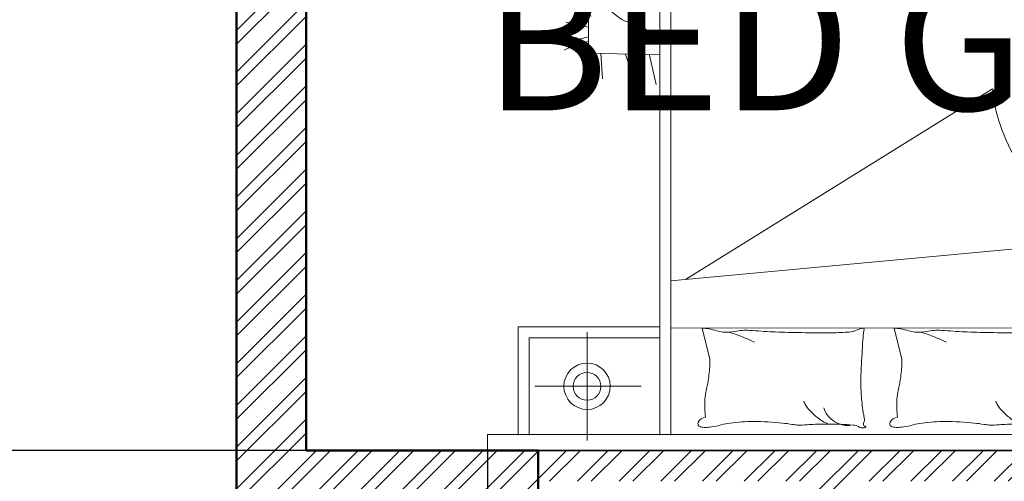
# Model space of a CAD drawing. Units: inches. Extents: x -90 to 536, y -553 to 299.
# Tile 17 of 27: x 10 to 137, y -2 to 58. Entities that reach past the tile are written whole.
import ezdxf

# ---------------------------------------------------------------- set-up
doc = ezdxf.new("R2010")
doc.units = ezdxf.units.IN
for name, color, linetype, lineweight in [('A-ANNO-DIMS', 2, 'Continuous', 18), ('A-WALL-PATT', 252, 'Continuous', 13), ('Furniture', 2, 'Continuous', 18), ('Inner Wall', 5, 'Continuous', 35), ('Outer Wall', 1, 'Continuous', 50)]:
    doc.layers.add(name, color=color, linetype=linetype, lineweight=lineweight)
doc.styles.get("Standard").update_dxf_attribs({"font": 'arial.ttf'})
doc.dimstyles.get("Standard").update_dxf_attribs({"dimtxt": 18, "dimasz": 12, "dimexe": 0.18, "dimexo": 0.0625, "dimgap": 0.09, "dimtad": 0, "dimtih": 1, "dimtoh": 1, "dimdec": 0, "dimzin": 0, "dimdsep": 46, "dimlunit": 3, "dimtxsty": 'Standard', "dimcen": 0.09, "dimadec": 0, "dimazin": 0, "dimtfac": 1, "dimtdec": 0, "dimtofl": 0, "dimtmove": 0, "dimatfit": 3, "dimfxl": 1, "dimtolj": 1, "dimtzin": 0, "dimarcsym": 0})

# ---------------------------------------------------------------- blocks, each defined once
blk = doc.blocks.new('A$C2B723114')
for p, q in [((0, 2.9047), (2.8274, 2.9047)), ((0, 2.8487), (0, 2.9047)), ((2.8274, 2.9047), (2.8274, 2.8487)), ((0.4243, 2.8697), (0.4243, 2.4855)), ((2.4742, 2.8697), (2.4742, 2.4855)), ((2.8274, 2.8487), (0, 2.8487)), ((0.1012, 2.4649), (0.1012, 2.849)), ((0.1396, 2.5033), (0.1396, 2.849)), ((0.6794, 0.7051), (0.6794, 2.8509)), ((0.7187, 0.7435), (0.7187, 2.8509)), ((2.1776, 2.8509), (2.1776, 0.7454)), ((2.216, 2.8509), (2.216, 0.707)), ((2.6798, 2.5052), (2.6798, 2.8509)), ((2.7182, 2.4668), (2.7182, 2.8509)), ((0.6087, 2.6776), (0.295, 2.6776)), ((2.6586, 2.6776), (2.2821, 2.6776)), ((1.3789, 2.4999), (1.3598, 2.5761)), ((2.0593, 2.4999), (2.0402, 2.5761)), ((0.6766, 2.5033), (0.1396, 2.5033)), ((1.3858, 2.4723), (1.3789, 2.4999)), ((2.0662, 2.4723), (2.0593, 2.4999)), ((2.2188, 2.5052), (2.6798, 2.5052)), ((0.6794, 2.4649), (0.1012, 2.4649)), ((0.7191, 2.47), (2.1778, 2.4719)), ((2.2188, 2.4668), (2.7182, 2.4668)), ((2.1771, 2.3036), (0.718, 2.1685)), ((1.0365, 1.6233), (2.1246, 2.2989)), ((2.2287, 1.6076), (2.2523, 1.5035)), ((0.5047, 1.5819), (0.5353, 1.4945)), ((0.6174, 1.5819), (0.6232, 1.4916)), ((0.6467, 1.5819), (0.6369, 1.5137)), ((0.6571, 1.4945), (0.6571, 1.5765)), ((2.2726, 1.593), (2.3061, 1.5007)), ((2.3067, 1.5881), (2.3373, 1.5007)), ((2.4194, 1.5881), (2.4251, 1.4979)), ((2.4487, 1.5881), (2.4389, 1.5199)), ((2.4591, 1.5007), (2.4591, 1.5828)), ((2.4685, 1.4964), (2.216, 1.5022)), ((0.4269, 0.0884), (0.4269, 1.4945)), ((0.4269, 1.4945), (0.6794, 1.4945)), ((2.4685, 1.4964), (2.4685, 0.0903)), ((2.4685, 1.4044), (2.5491, 1.3861)), ((0.3172, 1.3923), (0.4213, 1.3687)), ((2.4596, 1.3659), (2.552, 1.3324)), ((0.3318, 1.3485), (0.4241, 1.3149)), ((2.4645, 1.3318), (2.552, 1.3012)), ((0.3367, 1.3143), (0.4241, 1.2838)), ((2.4645, 1.2928), (2.5548, 1.2871)), ((2.4645, 1.2635), (2.5328, 1.2733)), ((2.4699, 1.2531), (2.552, 1.2163)), ((2.552, 1.2531), (2.4699, 1.2531)), ((2.5435, 1.2276), (2.4699, 1.2163)), ((0.3367, 1.2016), (0.427, 1.1959)), ((2.4699, 1.2163), (2.5463, 1.1823)), ((0.3367, 1.1724), (0.405, 1.1821)), ((0.4241, 1.162), (0.3421, 1.162)), ((0.3421, 1.162), (0.4241, 1.1252)), ((2.5491, 1.1654), (2.467, 1.1597)), ((2.5463, 1.1455), (2.467, 1.1342)), ((2.5491, 1.1342), (2.4699, 1.1201)), ((2.4699, 1.1201), (2.5491, 1.0946)), ((2.5463, 1.1172), (2.4727, 1.0918)), ((2.5491, 1.0946), (2.4699, 1.0635)), ((2.4699, 1.0635), (2.5491, 0.9842)), ((0.4157, 1.0206), (0.3421, 1.0093)), ((2.4642, 1.0267), (2.552, 0.9644)), ((0.3421, 1.0093), (0.4185, 0.9754)), ((2.4699, 0.9785), (2.552, 0.9531)), ((0.4213, 0.9584), (0.3392, 0.9527)), ((2.467, 0.9559), (2.552, 0.9333)), ((0.4185, 0.9386), (0.3392, 0.9272)), ((0.4213, 0.9272), (0.3421, 0.9131)), ((0.3421, 0.9131), (0.4213, 0.8876)), ((0.4185, 0.9103), (0.3449, 0.8848)), ((2.4642, 0.9389), (2.4869, 0.9276)), ((2.4869, 0.9276), (2.5265, 0.9163)), ((2.5265, 0.9163), (2.5491, 0.9163)), ((0.4213, 0.8876), (0.3421, 0.8565)), ((2.4642, 0.8908), (2.5152, 0.8483)), ((0.3421, 0.8565), (0.4213, 0.7772)), ((2.467, 0.8455), (2.5208, 0.8342)), ((2.5152, 0.8483), (2.5491, 0.837)), ((0.3364, 0.8197), (0.4241, 0.7574)), ((2.4699, 0.8172), (2.4925, 0.7974)), ((2.5491, 0.8087), (2.4699, 0.8172)), ((2.5208, 0.8342), (2.552, 0.8285)), ((2.552, 0.8285), (2.5293, 0.8087)), ((0.3421, 0.7716), (0.4241, 0.7461)), ((2.5491, 0.7606), (2.467, 0.7719)), ((2.4925, 0.7974), (2.535, 0.7889)), ((2.535, 0.7889), (2.552, 0.7861)), ((0.3392, 0.7489), (0.4241, 0.7263)), ((2.1776, 0.7454), (0.7187, 0.7435)), ((2.4727, 0.7464), (2.467, 0.7408)), ((2.552, 0.7464), (2.4727, 0.7464)), ((0.359, 0.7206), (0.3987, 0.7093)), ((0.3987, 0.7093), (0.4213, 0.7093)), ((2.216, 0.707), (0.6794, 0.7051)), ((0.9938, 0.6115), (1.7555, 0.7064)), ((2.467, 0.7153), (2.5491, 0.7238)), ((2.552, 0.7096), (2.467, 0.6842)), ((2.5491, 0.6842), (2.4642, 0.6615)), ((2.5491, 0.6672), (2.4755, 0.6587)), ((0.3421, 0.6601), (0.4213, 0.5808)), ((2.4755, 0.6474), (2.5548, 0.6276)), ((0.3364, 0.6233), (0.4241, 0.561)), ((2.4642, 0.6191), (2.4784, 0.6134)), ((2.467, 0.5993), (2.4869, 0.5964)), ((2.4784, 0.6134), (2.5406, 0.6077)), ((2.4869, 0.5964), (2.552, 0.5964)), ((2.5406, 0.6077), (2.552, 0.6134)), ((0.3421, 0.5752), (0.4241, 0.5497)), ((2.467, 0.5313), (2.5491, 0.5596)), ((0.3392, 0.5525), (0.4241, 0.5299)), ((0.359, 0.5242), (0.3987, 0.5129)), ((2.467, 0.5087), (2.5548, 0.5342)), ((2.5548, 0.5342), (2.4699, 0.4889)), ((1.4523, 0.5021), (1.1305, 0.4537)), ((0.3364, 0.4785), (0.3874, 0.436)), ((1.1305, 0.4537), (0.9938, 0.448)), ((0.3392, 0.4332), (0.393, 0.4219)), ((0.3874, 0.436), (0.4213, 0.4247)), ((0.393, 0.4219), (0.4241, 0.4162)), ((0.4213, 0.415), (0.3364, 0.3923)), ((0.4241, 0.2868), (0.3392, 0.415)), ((0.3421, 0.4049), (0.3647, 0.3851)), ((0.4213, 0.3964), (0.3421, 0.4049)), ((0.4213, 0.398), (0.3477, 0.3895)), ((0.3647, 0.3851), (0.4072, 0.3766)), ((0.4241, 0.4162), (0.4015, 0.3964)), ((2.467, 0.4133), (2.552, 0.4019)), ((2.467, 0.2879), (2.552, 0.4076)), ((0.4213, 0.3377), (0.3392, 0.3491)), ((0.4072, 0.3766), (0.4241, 0.3738)), ((0.4241, 0.3236), (0.3449, 0.3236)), ((2.467, 0.319), (2.5548, 0.3134)), ((0.3392, 0.2925), (0.4213, 0.3009)), ((2.4642, 0.3049), (2.5491, 0.2851)), ((0.3477, 0.2571), (0.427, 0.2373)), ((2.4699, 0.2491), (2.501, 0.2491)), ((2.501, 0.2491), (2.5491, 0.2547)), ((0.3506, 0.2231), (0.4128, 0.2175)), ((0.4128, 0.2175), (0.4241, 0.2231)), ((2.467, 0.2179), (2.5605, 0.1981)), ((0.359, 0.2061), (0.4241, 0.2061)), ((2.467, 0.1981), (2.5491, 0.1613)), ((2.467, 0.184), (2.4982, 0.1755)), ((2.4982, 0.1755), (2.5463, 0.1359)), ((0.3392, 0.1042), (0.4213, 0.1325)), ((0.3392, 0.0815), (0.427, 0.107)), ((0.427, 0.107), (0.3421, 0.0617)), ((2.4699, 0.1302), (2.535, 0.1104)), ((2.535, 0.1104), (2.5491, 0.0991)), ((2.4685, 0.0903), (0.4269, 0.0884)), ((0.5106, 0.094), (0.5106, 0.0657)), ((0.5417, 0.094), (0.5474, 0.0572)), ((0.587, 0.0884), (0.604, 0.0346)), ((0.6512, 0.0884), (0.6682, 0.0346)), ((0.713, 0.094), (0.713, 0.0657)), ((0.7334, 0.0943), (0.7503, 0.0434)), ((0.7786, 0.0915), (0.7786, 0.0632)), ((0.8739, 0.0884), (0.8908, 0.0346)), ((0.956, 0.0943), (0.973, 0.0434)), ((1.0013, 0.0915), (1.0013, 0.0632)), ((1.072, 0.0884), (1.089, 0.0346)), ((1.1338, 0.094), (1.1338, 0.0657)), ((1.1542, 0.0943), (1.1712, 0.0434)), ((1.1995, 0.0915), (1.1995, 0.0632)), ((1.4088, 0.094), (1.4088, 0.0657)), ((1.44, 0.094), (1.4456, 0.0572)), ((1.4853, 0.0884), (1.5023, 0.0346)), ((1.5674, 0.0962), (1.5844, 0.0453)), ((1.6127, 0.0934), (1.6127, 0.0651)), ((1.6297, 0.0849), (1.624, 0.0028)), ((1.6721, 0.0877), (1.6693, 0.0623)), ((1.7344, 0.0934), (1.7344, 0.0651)), ((1.7655, 0.0934), (1.7712, 0.0566)), ((1.8108, 0.0877), (1.8278, 0.034)), ((1.8568, 0.0962), (1.8738, 0.0453)), ((1.9342, 0.0962), (1.9512, 0.0453)), ((1.9795, 0.0934), (1.9795, 0.0651)), ((1.9965, 0.0849), (1.9908, 0.0028)), ((2.039, 0.0877), (2.0361, 0.0623)), ((2.1012, 0.0934), (2.1012, 0.0651)), ((2.1324, 0.0934), (2.138, 0.0566)), ((2.1777, 0.0877), (2.1946, 0.034)), ((2.2236, 0.0962), (2.2406, 0.0453)), ((2.2689, 0.0934), (2.2689, 0.0651)), ((2.2859, 0.0849), (2.2802, 0.0028)), ((2.3284, 0.0877), (2.3255, 0.0623)), ((2.3906, 0.0934), (2.3906, 0.0651)), ((2.4218, 0.0934), (2.4274, 0.0566)), ((2.4642, 0.0991), (2.5378, 0.0877)), ((2.467, 0.0877), (2.484, 0.034)), ((2.5378, 0.0877), (2.5463, 0.0821)), ((0.5106, 0.0657), (0.5077, 0.0063)), ((0.5474, 0.0572), (0.57, 0.0006)), ((0.713, 0.0657), (0.7101, 0.0063)), ((0.7503, 0.0434), (0.773, 0.0037)), ((0.7786, 0.0632), (0.7843, 0.0066)), ((0.973, 0.0434), (0.9957, 0.0037)), ((1.0013, 0.0632), (1.007, 0.0066)), ((1.1338, 0.0657), (1.131, 0.0063)), ((1.1712, 0.0434), (1.1939, 0.0037)), ((1.1995, 0.0632), (1.2052, 0.0066)), ((1.4088, 0.0657), (1.406, 0.0063)), ((1.4456, 0.0572), (1.4683, 0.0006)), ((1.5844, 0.0453), (1.607, 0.0057)), ((1.6127, 0.0651), (1.6184, 0.0085)), ((1.6693, 0.0623), (1.6608, 0.0028)), ((1.7344, 0.0651), (1.7316, 0.0057)), ((1.7712, 0.0566), (1.7938, 0)), ((1.8738, 0.0453), (1.8964, 0.0057)), ((1.9512, 0.0453), (1.9739, 0.0057)), ((1.9795, 0.0651), (1.9852, 0.0085)), ((2.0361, 0.0623), (2.0276, 0.0028)), ((2.1012, 0.0651), (2.0984, 0.0057)), ((2.138, 0.0566), (2.1607, 0)), ((2.2406, 0.0453), (2.2632, 0.0057)), ((2.2689, 0.0651), (2.2746, 0.0085)), ((2.3255, 0.0623), (2.317, 0.0028)), ((2.3906, 0.0651), (2.3878, 0.0057)), ((2.4274, 0.0566), (2.4501, 0)), ((0.604, 0.0346), (0.621, 0.0063)), ((0.6682, 0.0346), (0.6851, 0.0063)), ((0.8908, 0.0346), (0.9078, 0.0063)), ((1.089, 0.0346), (1.106, 0.0063)), ((1.5023, 0.0346), (1.5192, 0.0082)), ((1.8278, 0.034), (1.8448, 0.0057)), ((2.1946, 0.034), (2.2116, 0.0057)), ((2.484, 0.034), (2.501, 0.0057))]:
    blk.add_line(p, q)
for centre, radius in [((0.4243, 2.6776), 0.0821), ((2.4742, 2.6776), 0.0821), ((0.4243, 2.6776), 0.0493), ((2.4742, 2.6776), 0.0493)]:
    blk.add_circle(centre, radius)
for centre, radius, start, end in [((0.8078, 2.821), 0.00214, 160.436, 281.8931), ((0.8088, 2.8207), 0.00315, 111.7883, 160.436), ((0.8162, 2.8021), 0.0232, 94.3025, 111.7883), ((0.8091, 2.8151), 0.00394, 21.9904, 101.8931), ((0.8409, 2.7949), 0.0302, 158.579, 188.1335), ((0.7994, 2.8112), 0.0144, 338.579, 21.9904), ((0.8165, 2.7987), 0.0266, 59.3487, 94.3025), ((0.8554, 2.8643), 0.0497, 239.3487, 264.7408), ((0.9202, 3.5684), 0.7568, 264.7408, 268.0921), ((0.8679, 2.7254), 0.0915, 74.0648, 94.2159), ((0.8679, 2.7254), 0.0915, 53.9136, 74.0648), ((0.9409, 4.189), 1.3777, 268.0921, 270.5757), ((0.8679, 2.7254), 0.0915, 36.1766, 53.9136), ((0.86, 2.6097), 0.2158, 62.7604, 69.1397), ((0.9466, 3.6164), 0.8051, 270.5757, 274.8018), ((0.9263, 2.7386), 0.0708, 51.6114, 62.7604), ((0.7461, 2.511), 0.3611, 46.1885, 51.6114), ((1.0364, 2.548), 0.2671, 87.4614, 94.8018), ((1.042, 2.6745), 0.1405, 79.8101, 87.4614), ((1.1532, 3.2931), 0.488, 259.8101, 263.9133), ((1.204, 3.7695), 0.9671, 263.9133, 270), ((1.204, 3.4318), 0.6294, 270, 277.5469), ((1.2573, 3.0292), 0.2233, 277.5469, 285.744), ((1.3941, 2.5438), 0.281, 98.4372, 105.744), ((1.3747, 2.6748), 0.1486, 90, 98.4372), ((1.3713, 2.8186), 0.0315, 274.4002, 333.4195), ((1.3747, 2.74), 0.0833, 78.7276, 90), ((1.3886, 2.8099), 0.0121, 333.4195, 78.7276), ((1.4882, 2.821), 0.00214, 160.436, 281.8931), ((1.4892, 2.8207), 0.00315, 111.7883, 160.436), ((1.4966, 2.8021), 0.0232, 94.3025, 111.7883), ((1.4895, 2.8151), 0.00394, 21.9904, 101.8931), ((1.5213, 2.7949), 0.0302, 158.579, 188.1335), ((1.4798, 2.8112), 0.0144, 338.579, 21.9904), ((1.4969, 2.7987), 0.0266, 59.3487, 94.3025), ((1.5358, 2.8643), 0.0497, 239.3487, 264.7408), ((1.6006, 3.5684), 0.7568, 264.7408, 268.0921), ((1.5483, 2.7254), 0.0915, 74.0648, 94.2159), ((1.5483, 2.7254), 0.0915, 53.9136, 74.0648), ((1.6213, 4.189), 1.3777, 268.0921, 270.5757), ((1.5483, 2.7254), 0.0915, 36.1766, 53.9136), ((1.5404, 2.6097), 0.2158, 62.7604, 69.1397), ((1.627, 3.6164), 0.8051, 270.5757, 274.8018), ((1.6067, 2.7386), 0.0708, 51.6114, 62.7604), ((1.4265, 2.511), 0.3611, 46.1885, 51.6114), ((1.7168, 2.548), 0.2671, 87.4614, 94.8018), ((1.7224, 2.6745), 0.1405, 79.8101, 87.4614), ((1.8336, 3.2931), 0.488, 259.8101, 263.9133), ((1.8844, 3.7695), 0.9671, 263.9133, 270), ((1.8844, 3.4318), 0.6294, 270, 277.5469), ((1.9377, 3.0292), 0.2233, 277.5469, 285.744), ((2.0745, 2.5438), 0.281, 98.4372, 105.744), ((2.0551, 2.6748), 0.1486, 90, 98.4372), ((2.0517, 2.8186), 0.0315, 274.4002, 333.4195), ((2.0551, 2.74), 0.0833, 78.7276, 90), ((2.069, 2.8099), 0.0121, 333.4195, 78.7276), ((1.0356, 2.8227), 0.2268, 188.1335, 192.1095), ((0.635, 2.7368), 0.1829, 7.6809, 12.1095), ((-0.0181, 2.6487), 0.8418, 3.3687, 7.6809), ((0.8679, 2.7254), 0.0915, 18.4397, 36.1766), ((0.8523, 2.6218), 0.2076, 39.0349, 46.1885), ((0.923, 2.7382), 0.4535, 0, 6.2324), ((1.716, 2.8227), 0.2268, 188.1335, 192.1095), ((1.3154, 2.7368), 0.1829, 7.6809, 12.1095), ((0.6623, 2.6487), 0.8418, 3.3687, 7.6809), ((1.5483, 2.7254), 0.0915, 18.4397, 36.1766), ((1.5327, 2.6218), 0.2076, 39.0349, 46.1885), ((1.6034, 2.7382), 0.4535, 0, 6.2324), ((0.9783, 2.7239), 0.0455, 28.3168, 39.0349), ((0.8558, 2.6579), 0.1846, 23.0028, 28.3168), ((1.1884, 2.7382), 0.1881, 350.3156, 0), ((1.6587, 2.7239), 0.0455, 28.3168, 39.0349), ((1.5362, 2.6579), 0.1846, 23.0028, 28.3168), ((1.8688, 2.7382), 0.1881, 350.3156, 0), ((0.1976, 2.6614), 0.6258, 358.3669, 3.3687), ((0.5722, 2.8434), 0.8132, 347.8016, 350.3156), ((0.878, 2.6614), 0.6258, 358.3669, 3.3687), ((1.2526, 2.8434), 0.8132, 347.8016, 350.3156), ((1.6528, 2.6098), 0.2924, 167.8016, 171.9949), ((2.3332, 2.6098), 0.2924, 167.8016, 171.9949), ((-0.4351, 2.6794), 1.2587, 356.945, 358.3669), ((1.9648, 2.5659), 0.6074, 171.9949, 177.3351), ((0.2453, 2.6794), 1.2587, 356.945, 358.3669), ((2.6452, 2.5659), 0.6074, 171.9949, 177.3351), ((-11.7321, 3.2823), 12.5718, 356.49514, 356.94504), ((1.4204, 2.5912), 0.0624, 177.3351, 194.0452), ((-11.0517, 3.2823), 12.5718, 356.49514, 356.94504), ((2.1008, 2.5912), 0.0624, 177.3351, 194.0452), ((0.5206, 2.5319), 0.2961, 350.0016, 356.4951), ((1.4917, 3.1364), 0.681, 244.6889, 246.5156), ((1.201, 2.5319), 0.2961, 350.0016, 356.4951), ((2.1721, 3.1364), 0.681, 244.6889, 246.5156), ((0.8298, 2.4774), 0.0178, 170.0016, 196.6978), ((0.8068, 2.5419), 0.0707, 286.2212, 297.2841), ((0.8584, 2.4419), 0.0418, 102.869, 117.2841), ((0.879, 2.3515), 0.1345, 93.574, 102.869), ((0.9376, 1.4146), 1.0732, 90.2865, 93.574), ((0.9586, -2.7845), 5.2724, 89.0296, 90.2865), ((0.9954, -0.6123), 3.0999, 87.3904, 89.0296), ((1.0854, 1.364), 1.1216, 85.3824, 87.3904), ((1.28, 3.7729), 1.2952, 265.3824, 267.2509), ((1.228, 2.691), 0.2121, 267.2509, 281.5586), ((1.4917, 3.1364), 0.681, 246.5156, 248.3423), ((1.4917, 3.1364), 0.681, 248.3423, 250.572), ((1.4917, 3.1364), 0.681, 250.572, 252.8018), ((1.2975, 2.3514), 0.1345, 83.5659, 101.5586), ((1.3002, 2.3754), 0.1104, 72.6136, 83.5659), ((1.3965, 2.6828), 0.2118, 252.6136, 260.5159), ((1.5102, 2.4774), 0.0178, 170.0016, 196.6978), ((1.4872, 2.5419), 0.0707, 286.2212, 297.2841), ((1.5388, 2.4419), 0.0418, 102.869, 117.2841), ((1.5594, 2.3515), 0.1345, 93.574, 102.869), ((1.618, 1.4146), 1.0732, 90.2865, 93.574), ((1.639, -2.7845), 5.2724, 89.0296, 90.2865), ((1.6758, -0.6123), 3.0999, 87.3904, 89.0296), ((1.7658, 1.364), 1.1216, 85.3824, 87.3904), ((1.9604, 3.7729), 1.2952, 265.3824, 267.2509), ((1.9084, 2.691), 0.2121, 267.2509, 281.5586), ((2.1721, 3.1364), 0.681, 246.5156, 248.3423), ((2.1721, 3.1364), 0.681, 248.3423, 250.572), ((2.1721, 3.1364), 0.681, 250.572, 252.8018), ((1.9779, 2.3514), 0.1345, 83.5659, 101.5586), ((1.9806, 2.3754), 0.1104, 72.6136, 83.5659), ((2.0769, 2.6828), 0.2118, 252.6136, 260.5159), ((0.8139, 2.4726), 0.00122, 196.6978, 277.1204), ((0.8041, 2.5514), 0.0807, 277.1204, 286.2212), ((1.4027, 2.7202), 0.2496, 260.5159, 265.9171), ((1.385, 2.4721), 0.000845, 265.9171, 14.0449), ((1.4943, 2.4726), 0.00122, 196.6978, 277.1204), ((1.4845, 2.5514), 0.0807, 277.1204, 286.2212), ((2.0831, 2.7202), 0.2496, 260.5159, 265.9171), ((2.0654, 2.4721), 0.000845, 265.9171, 14.0449)]:
    blk.add_arc(centre, radius, start, end)
blk.add_ellipse((0.4962, 1.9132), major_axis=(0.4887, -0.4605), ratio=0.503305, start_param=0.491272, end_param=1.591113)
for points, knots in [([(0.427, 1.4678), (0.4036, 1.4582), (0.3693, 1.4441), (0.3335, 1.4344), (0.3221, 1.4313)], [0, 0, 0, 0, 98.452083, 144.639601, 144.639601, 144.639601, 144.639601]), ([(0.6768, 1.3104), (0.6615, 1.3339), (0.6315, 1.3797), (0.604, 1.4501), (0.5417, 1.4748), (0.5064, 1.4871), (0.4848, 1.4945)], [0, 0, 0, 0, 110.980521, 216.571322, 273.316778, 363.252298, 363.252298, 363.252298, 363.252298]), ([(2.5548, 1.4853), (2.5314, 1.4757), (2.5031, 1.4641), (2.4737, 1.4555), (2.4685, 1.454)], [0, 0, 0, 0, 98.452083, 119.481049, 119.481049, 119.481049, 119.481049]), ([(0.4241, 1.4423), (0.4031, 1.437), (0.3691, 1.4284), (0.3351, 1.4199), (0.3221, 1.4167)], [0, 0, 0, 0, 84.638756, 136.955563, 136.955563, 136.955563, 136.955563]), ([(2.552, 1.4598), (2.5309, 1.4545), (2.5031, 1.4475), (2.4753, 1.4406), (2.4685, 1.4389)], [0, 0, 0, 0, 84.638756, 111.94623, 111.94623, 111.94623, 111.94623]), ([(2.2145, 1.4211), (2.233, 1.4246), (2.2636, 1.4303), (2.2761, 1.3837), (2.3429, 1.3967), (2.3949, 1.3342), (2.4474, 1.3031), (2.4698, 1.2898)], [0, 0, 0, 0, 61.886907, 102.717887, 145.699352, 284.082577, 386.765171, 386.765171, 386.765171, 386.765171]), ([(0.6768, 1.286), (0.6567, 1.2911), (0.6145, 1.3017), (0.5543, 1.3533), (0.4816, 1.349), (0.4362, 1.3493), (0.4233, 1.3493)], [0, 0, 0, 0, 80.250278, 168.388677, 295.908361, 346.663112, 346.663112, 346.663112, 346.663112]), ([(0.4233, 1.3445), (0.4367, 1.3385), (0.464, 1.3264), (0.5129, 1.2848), (0.5456, 1.2161), (0.6131, 1.2349), (0.6142, 1.1913), (0.6642, 1.1806), (0.674, 1.144), (0.6817, 1.1154)], [0, 0, 0, 0, 56.745495, 115.23739, 254.956954, 286.678662, 337.828324, 366.201072, 468.500395, 468.500395, 468.500395, 468.500395]), ([(2.2145, 1.319), (2.2295, 1.319), (2.2678, 1.3192), (2.3288, 1.2705), (2.4143, 1.279), (2.4535, 1.2403), (2.4662, 1.2278)], [0, 0, 0, 0, 57.155505, 146.33427, 287.936209, 355.396728, 355.396728, 355.396728, 355.396728]), ([(2.3573, 1.127), (2.3656, 1.1759), (2.3758, 1.2352), (2.3371, 1.1853), (2.3602, 1.1713), (2.3768, 1.1612)], [0, 0, 0, 0, 107.853607, 130.728419, 189.220329, 189.220329, 189.220329, 189.220329]), ([(2.2182, 1.2059), (2.2419, 1.1958), (2.3116, 1.1659), (2.342, 1.0552), (2.4266, 1.0223), (2.4474, 0.9811), (2.462, 0.9684), (2.4698, 0.9616)], [0, 0, 0, 0, 97.73655, 287.59661, 389.176293, 423.403759, 463.679181, 463.679181, 463.679181, 463.679181]), ([(2.2145, 1.1476), (2.2246, 1.1286), (2.2575, 1.0666), (2.3612, 1.0009), (2.431, 0.9336), (2.4662, 0.8996)], [0, 0, 0, 0, 83.02987, 271.460712, 463.033803, 463.033803, 463.033803, 463.033803]), ([(0.6817, 0.8034), (0.6673, 0.8119), (0.6341, 0.8315), (0.5785, 0.8518), (0.5349, 0.8973), (0.4828, 0.9461), (0.4518, 0.9879), (0.4331, 1.013)], [0, 0, 0, 0, 65.318952, 150.437229, 226.833166, 307.58338, 429.454095, 429.454095, 429.454095, 429.454095]), ([(0.4282, 0.9448), (0.4547, 0.9353), (0.496, 0.9206), (0.5223, 0.8436), (0.5628, 0.7946), (0.6113, 0.7575), (0.6214, 0.7173), (0.6539, 0.7022), (0.672, 0.6897), (0.6768, 0.6864)], [0, 0, 0, 0, 102.299436, 159.044876, 303.717955, 348.579152, 391.138254, 454.581655, 477.456496, 477.456496, 477.456496, 477.456496]), ([(2.2145, 0.823), (2.227, 0.8201), (2.261, 0.8121), (2.261, 0.7401), (2.3352, 0.7659), (2.379, 0.6836), (2.4336, 0.6521), (2.4662, 0.6334)], [0, 0, 0, 0, 46.747668, 127.438174, 179.649794, 280.561838, 429.605131, 429.605131, 429.605131, 429.605131]), ([(0.4282, 0.74), (0.4347, 0.7029), (0.444, 0.6496), (0.5194, 0.6274), (0.555, 0.5807), (0.5975, 0.5243), (0.6789, 0.5415), (0.677, 0.5095), (0.6768, 0.5061)], [0, 0, 0, 0, 130.791737, 187.537266, 286.231946, 353.673191, 460.023761, 472.712403, 472.712403, 472.712403, 472.712403]), ([(2.2218, 0.7246), (2.2595, 0.716), (2.3548, 0.6945), (2.4265, 0.6268), (2.4698, 0.586)], [0, 0, 0, 0, 148.665024, 375.555892, 375.555892, 375.555892, 375.555892]), ([(2.3719, 0.6737), (2.3738, 0.6431), (2.3772, 0.5878), (2.3146, 0.6382), (2.3401, 0.7015), (2.2971, 0.6649), (2.2923, 0.6965), (2.289, 0.7176)], [0, 0, 0, 0, 83.446591, 150.887818, 201.642461, 230.015204, 286.760644, 286.760644, 286.760644, 286.760644]), ([(0.6768, 0.6864), (0.7275, 0.655), (0.8251, 0.5944), (0.9391, 0.606), (0.9938, 0.6115)], [0, 0, 0, 0, 225.995823, 434.686543, 434.686543, 434.686543, 434.686543]), ([(2.2145, 0.5167), (2.1764, 0.5522), (2.1051, 0.6184), (1.9357, 0.5803), (1.9385, 0.6342), (1.9388, 0.6395)], [0, 0, 0, 0, 208.073343, 389.01094, 409.01094, 409.01094, 409.01094, 409.01094]), ([(0.6768, 0.5061), (0.7554, 0.4794), (0.8591, 0.4442), (0.9675, 0.4473), (0.9938, 0.448)], [0, 0, 0, 0, 319.374611, 421.61723, 421.61723, 421.61723, 421.61723]), ([(0.4331, 0.4427), (0.4498, 0.4356), (0.4827, 0.4216), (0.5314, 0.3759), (0.632, 0.3884), (0.6996, 0.3513), (0.7423, 0.3278)], [0, 0, 0, 0, 70.931849, 139.556414, 248.154027, 434.709995, 434.709995, 434.709995, 434.709995]), ([(2.4625, 0.1088), (2.4095, 0.1438), (2.2904, 0.2226), (2.0623, 0.1771), (1.9006, 0.2246), (1.7699, 0.2337), (1.6941, 0.2766), (1.5528, 0.2786), (1.4005, 0.2587), (1.2324, 0.3267), (1.059, 0.2939), (0.9218, 0.426), (0.7359, 0.3204), (0.5586, 0.2391), (0.4502, 0.3116), (0.427, 0.3272)], [0, 0, 0, 0, 239.874704, 538.942419, 850.40885, 893.390315, 1047.998294, 1176.505142, 1437.500972, 1637.333004, 1864.324391, 2089.058767, 2248.736533, 2637.953392, 2744.252142, 2744.252142, 2744.252142, 2744.252142]), ([(1.9771, 0.0962), (1.9286, 0.1117), (1.7864, 0.157), (1.5223, 0.1992), (1.2611, 0.141), (1.0527, 0.2023), (0.8859, 0.1885), (0.76, 0.3042), (0.6211, 0.292), (0.5187, 0.3203), (0.4572, 0.3456), (0.4282, 0.3575)], [0, 0, 0, 0, 198.710624, 582.73994, 1031.873213, 1206.082894, 1423.278209, 1655.952104, 1808.744089, 1945.69963, 2068.229211, 2068.229211, 2068.229211, 2068.229211]), ([(0.8718, 0.2941), (0.8821, 0.3221), (0.9041, 0.3814), (0.9523, 0.2773), (0.8733, 0.2454), (0.8757, 0.2798), (0.8766, 0.2941)], [0, 0, 0, 0, 82.720021, 175.094899, 237.579423, 282.440623, 282.440623, 282.440623, 282.440623]), ([(0.8474, 0.0943), (0.82, 0.1047), (0.757, 0.1287), (0.6201, 0.1029), (0.4623, 0.1837), (0.4372, 0.2936), (0.4282, 0.3331)], [0, 0, 0, 0, 112.422038, 258.341957, 533.791494, 688.286079, 688.286079, 688.286079, 688.286079]), ([(1.2715, 0.221), (1.3344, 0.2172), (1.4529, 0.21), (1.2971, 0.2665), (1.2756, 0.2284), (1.2715, 0.221)], [0, 0, 0, 0, 150.888188, 283.977876, 315.699589, 315.699589, 315.699589, 315.699589])]:
    blk.add_open_spline(points, degree=3, knots=knots)
blk = doc.blocks.new('*D33')
at = {"layer": 'A-ANNO-DIMS', "color": 0, "lineweight": -2, "transparency": 16777216}
for p, q in [((173.76, 108.4), (189.77, 108.4)), ((189.59, 96.4), (189.59, 64.83)), ((189.59, 14.45), (189.59, 46.02)), ((173.76, 2.45), (189.77, 2.45))]:
    blk.add_line(p, q, dxfattribs=at)
at = {"layer": 'A-ANNO-DIMS', "color": 0, "transparency": 16777216}
for points in [[(187.59, 96.4), (191.59, 96.4), (189.59, 108.4)], [(187.59, 14.45), (191.59, 14.45), (189.59, 2.45)]]:
    blk.add_solid(points, dxfattribs=at)
at = {"layer": 'Defpoints', "color": 0, "transparency": 16777216}
for p in [(173.7, 108.4), (173.7, 2.45), (189.59, 2.45)]:
    blk.add_point(p, dxfattribs=at)
at = {"layer": 'A-ANNO-DIMS', "color": 0, "transparency": 16777216, "insert": (189.59, 55.42), "char_height": 18, "attachment_point": 5}
blk.add_mtext('\\A1;BED GROUP 106 TYP.', dxfattribs=at)
blk = doc.blocks.new('*D34')
at = {"layer": 'A-ANNO-DIMS', "color": 0, "lineweight": -2, "transparency": 16777216}
for p, q in [((70.57, 2.38), (70.57, -13.63)), ((173.7, 2.38), (173.7, -13.63)), ((58.57, -13.45), (46.57, -13.45)), ((185.7, -13.45), (197.7, -13.45))]:
    blk.add_line(p, q, dxfattribs=at)
at = {"layer": 'A-ANNO-DIMS', "color": 0, "transparency": 16777216}
for points in [[(58.57, -11.45), (58.57, -15.45), (70.57, -13.45)], [(185.7, -11.45), (185.7, -15.45), (173.7, -13.45)]]:
    blk.add_solid(points, dxfattribs=at)
at = {"layer": 'Defpoints', "color": 0, "transparency": 16777216}
for p in [(70.57, 2.45), (173.7, 2.45), (70.57, -13.45)]:
    blk.add_point(p, dxfattribs=at)
at = {"layer": 'A-ANNO-DIMS', "color": 0, "transparency": 16777216, "insert": (122.13, -13.45), "char_height": 18, "attachment_point": 5}
blk.add_mtext('\\A1;103 TYP.', dxfattribs=at)
blk = doc.blocks.new('*D53')
at = {"layer": 'A-ANNO-DIMS', "color": 0, "lineweight": -2, "transparency": 16777216}
for p, q in [((35.09, 103.75), (35.09, 287.38)), ((47.09, 287.2), (183.7, 287.2)), ((395.13, 287.2), (258.52, 287.2)), ((407.13, -63.49), (407.13, 287.38))]:
    blk.add_line(p, q, dxfattribs=at)
at = {"layer": 'A-ANNO-DIMS', "color": 0, "transparency": 16777216}
for points in [[(47.09, 289.2), (47.09, 285.2), (35.09, 287.2)], [(395.13, 289.2), (395.13, 285.2), (407.13, 287.2)]]:
    blk.add_solid(points, dxfattribs=at)
at = {"layer": 'Defpoints', "color": 0, "transparency": 16777216}
for p in [(407.13, 287.2), (35.09, 103.69), (407.13, -63.55)]:
    blk.add_point(p, dxfattribs=at)
at = {"layer": 'A-ANNO-DIMS', "color": 0, "transparency": 16777216, "insert": (221.11, 287.2), "char_height": 18, "attachment_point": 5}
blk.add_mtext('\\A1;372.04', dxfattribs=at)
blk = doc.blocks.new('*D54')
at = {"layer": 'A-ANNO-DIMS', "color": 0, "lineweight": -2, "transparency": 16777216}
for p, q in [((113.07, 249.45), (-2.85, 249.45)), ((-2.67, 237.45), (-2.67, -117.77)), ((-2.67, -491.55), (-2.67, -136.34)), ((38.07, -503.55), (-2.85, -503.55))]:
    blk.add_line(p, q, dxfattribs=at)
at = {"layer": 'A-ANNO-DIMS', "color": 0, "transparency": 16777216}
for points in [[(-4.67, 237.45), (-0.67, 237.45), (-2.67, 249.45)], [(-4.67, -491.55), (-0.67, -491.55), (-2.67, -503.55)]]:
    blk.add_solid(points, dxfattribs=at)
at = {"layer": 'Defpoints', "color": 0, "transparency": 16777216}
for p in [(-2.67, 249.45), (113.13, 249.45), (38.13, -503.55)]:
    blk.add_point(p, dxfattribs=at)
at = {"layer": 'A-ANNO-DIMS', "color": 0, "transparency": 16777216, "insert": (-2.67, -127.05), "char_height": 18, "attachment_point": 5}
blk.add_mtext('\\A1;753', dxfattribs=at)
blk = doc.blocks.new('*D56')
at = {"layer": 'A-ANNO-DIMS', "color": 0, "lineweight": -2, "transparency": 16777216}
for p, q in [((47.07, 134.45), (-2.85, 134.45)), ((-2.67, 122.45), (-2.67, 77.73)), ((-2.67, 14.45), (-2.67, 59.16)), ((47.07, 2.45), (-2.85, 2.45))]:
    blk.add_line(p, q, dxfattribs=at)
at = {"layer": 'A-ANNO-DIMS', "color": 0, "transparency": 16777216}
for points in [[(-4.67, 122.45), (-0.67, 122.45), (-2.67, 134.45)], [(-4.67, 14.45), (-0.67, 14.45), (-2.67, 2.45)]]:
    blk.add_solid(points, dxfattribs=at)
at = {"layer": 'Defpoints', "color": 0, "transparency": 16777216}
for p in [(-2.67, 134.45), (47.13, 134.45), (47.13, 2.45)]:
    blk.add_point(p, dxfattribs=at)
at = {"layer": 'A-ANNO-DIMS', "color": 0, "transparency": 16777216, "insert": (-2.67, 68.45), "char_height": 18, "attachment_point": 5}
blk.add_mtext('\\A1;132', dxfattribs=at)

msp = doc.modelspace()

# ---------------------------------------------------------------- hatches: boundary and pattern name
at = {"layer": 'A-WALL-PATT'}
h = msp.add_hatch(dxfattribs=at)
h.set_pattern_fill('ANSI32', color=256, scale=0.4)
h.set_pattern_definition([(45, (-88.8105, -603.6155), (-2.694077, 2.694077), []), (45, (-87.0145, -603.6155), (-2.694077, 2.694077), [])])
h.paths.add_polyline_path([(285.1317, 246.4462), (131.1317, 246.4462), (131.1317, 237.4462), (285.1317, 237.4462)])
h.paths.add_polyline_path([(122.1317, 237.4462), (113.1317, 237.4462), (113.1317, 152.4462), (122.1317, 152.4462), (122.1317, 166.4704)])
h.paths.add_polyline_path([(303.1317, 237.4462), (294.1317, 237.4462), (294.1317, 152.4462), (303.1317, 152.4462)])
h.paths.add_polyline_path([(47.1317, 91.9277), (38.1317, 91.9277), (38.1317, -6.5538), (77.1317, -6.5538), (77.1317, 2.4462), (70.5655, 2.4462), (47.1317, 2.4462)])
h.paths.add_polyline_path([(83.052, -61.5538), (47.1317, -61.5538), (47.1317, -24.5538), (38.1317, -24.5538), (38.1317, -70.5538), (74.052, -70.5538), (74.052, -223.5538), (38.1317, -223.5538), (38.1317, -503.5538), (92.1317, -503.5538), (92.1317, -437.5538), (191.1317, -437.5538), (191.1317, -428.5538), (83.1317, -428.5538), (83.1317, -494.5538), (47.1317, -494.5538), (47.1317, -232.5538), (83.052, -232.5538), (83.052, -70.5538)])
h.paths.add_polyline_path([(407.1317, -63.5538), (381.1317, -63.5538), (381.1317, 91.9277), (372.1317, 91.9277), (372.1317, 32.8805), (372.1317, -63.5538), (306.5745, -63.5538), (237.1317, -63.5538), (237.1317, -38.5538), (233.1317, -38.5538), (233.1317, -71.5538), (398.1317, -71.5538), (398.1317, -152.5538), (233.1317, -152.5538), (233.1317, -161.5538), (398.1317, -161.5538), (398.1317, -368.5538), (233.1317, -368.5538), (233.1317, -377.5538), (407.1317, -377.5538), (407.1317, -161.5538)])
h.paths.add_polyline_path([(261.1317, -422.5538), (252.1317, -422.5538), (252.1317, -428.5538), (233.1317, -428.5538), (233.1317, -437.5538), (261.1317, -437.5538)])
h.paths.add_polyline_path([(191.1317, -368.5538), (180.1317, -368.5538), (180.1317, -335.5538), (131.5919, -335.5538), (131.5919, -344.5538), (171.1317, -344.5538), (171.1317, -392.5538), (180.1317, -392.5538), (180.1317, -377.5538), (191.1317, -377.5538)], flags=17)
h.paths.add_polyline_path([(180.1317, -223.5538), (152.1317, -223.5538), (152.1317, -227.5538), (176.1317, -227.5538), (176.1317, -335.5538), (180.1317, -335.5538)], flags=17)
h.paths.add_polyline_path([(131.5919, -335.5538), (83.1317, -335.5538), (83.1317, -339.5538), (83.1317, -392.5538), (87.1317, -392.5538), (87.1317, -339.5538), (131.5919, -339.5538)], flags=17)
h.paths.add_polyline_path([(197.1317, 2.4462), (77.1317, 2.4462), (77.1317, -1.5538), (113.1317, -1.5538), (113.1317, -71.5538), (181.1317, -71.5538), (181.1317, -67.5538), (117.1317, -67.5538), (117.1317, -1.5538), (177.1317, -1.5538), (177.1317, -37.5538), (181.1317, -37.5538), (181.1317, -1.5538), (197.1317, -1.5538)])
h.paths.add_polyline_path([(173.1317, 138.4462), (122.1317, 138.4462), (122.1317, 134.4462), (173.1317, 134.4462)])
h.paths.add_polyline_path([(213.1317, 237.4462), (209.1317, 237.4462), (209.1317, 134.4462), (233.1317, 134.4462), (233.1317, 68.8889), (233.1317, -2.5538), (237.1317, -2.5538), (237.1317, 134.4462), (258.1317, 134.4462), (258.1317, 138.4462), (213.1317, 138.4462)])

# ---------------------------------------------------------------- linework, layer by layer
at = {"layer": 'Inner Wall'}
msp.add_line((197.1317, 2.4462), (47.1317, 2.4462), dxfattribs=at)
at = {"layer": 'Outer Wall'}
for p, q in [((47.1317, 103.6916), (47.1317, 2.4462)), ((38.1317, 91.9277), (38.1317, -6.5538)), ((47.1317, 2.4462), (77.1317, 2.4462)), ((77.1317, 2.4462), (77.1317, -6.5538))]:
    msp.add_line(p, q, dxfattribs=at)

# ---------------------------------------------------------------- block references
at = {"layer": 'Furniture', "xscale": 36.47664764473289, "yscale": 36.47664764473289, "zscale": 36.47664764473289, "rotation": 180}
msp.add_blockref('A$C2B723114', (173.698, 108.4009), dxfattribs=at)

# ---------------------------------------------------------------- dimensions: what is measured, and where the dimension line sits
at = {"layer": 'A-ANNO-DIMS'}
dim = msp.add_linear_dim(base=(407.1317, 287.2012), p1=(35.0873, 103.6916), p2=(407.1317, -63.5538), dimstyle='Standard', override={"dimdec": 2, "dimlfac": 1, "dimrnd": 0, "dimzin": 0, "dimdsep": 46, "dimlunit": 2}, dxfattribs=at)
dim.commit()
dim.dimension.update_dxf_attribs({"geometry": '*D53', "text_midpoint": (221.1095, 287.2012)})
for base, p1, p2, picture, middle in [((-2.6677, 249.4462), (38.1317, -503.5538), (113.1317, 249.4462), '*D54', (-2.6677, -127.0538)), ((-2.6677, 134.4462), (47.1317, 2.4462), (47.1317, 134.4462), '*D56', (-2.6677, 68.4462))]:
    dim = msp.add_linear_dim(base=base, p1=p1, p2=p2, angle=90, dimstyle='Standard', override={"dimdec": 0, "dimlfac": 1, "dimrnd": 0, "dimzin": 0, "dimdsep": 46, "dimlunit": 2}, dxfattribs=at)
    dim.commit()
    dim.dimension.update_dxf_attribs({"geometry": picture, "text_midpoint": middle})
for base, p1, p2, angle, text, picture, middle in [((189.5912, 2.4462), (173.698, 108.4009), (173.698, 2.4462), 270, 'BED GROUP <> TYP.', '*D33', (189.5912, 55.4235)), ((70.5655, -13.447), (173.698, 2.4462), (70.5655, 2.4462), 180, '<> TYP.', '*D34', (122.1317, -13.447))]:
    dim = msp.add_linear_dim(base=base, p1=p1, p2=p2, angle=angle, text=text, dimstyle='Standard', override={"dimdec": 0, "dimlfac": 1, "dimrnd": 0, "dimzin": 0, "dimdsep": 46, "dimlunit": 2}, dxfattribs=at)
    dim.commit()
    dim.dimension.update_dxf_attribs({"geometry": picture, "text_midpoint": middle})

doc.saveas('drawing.dxf')
